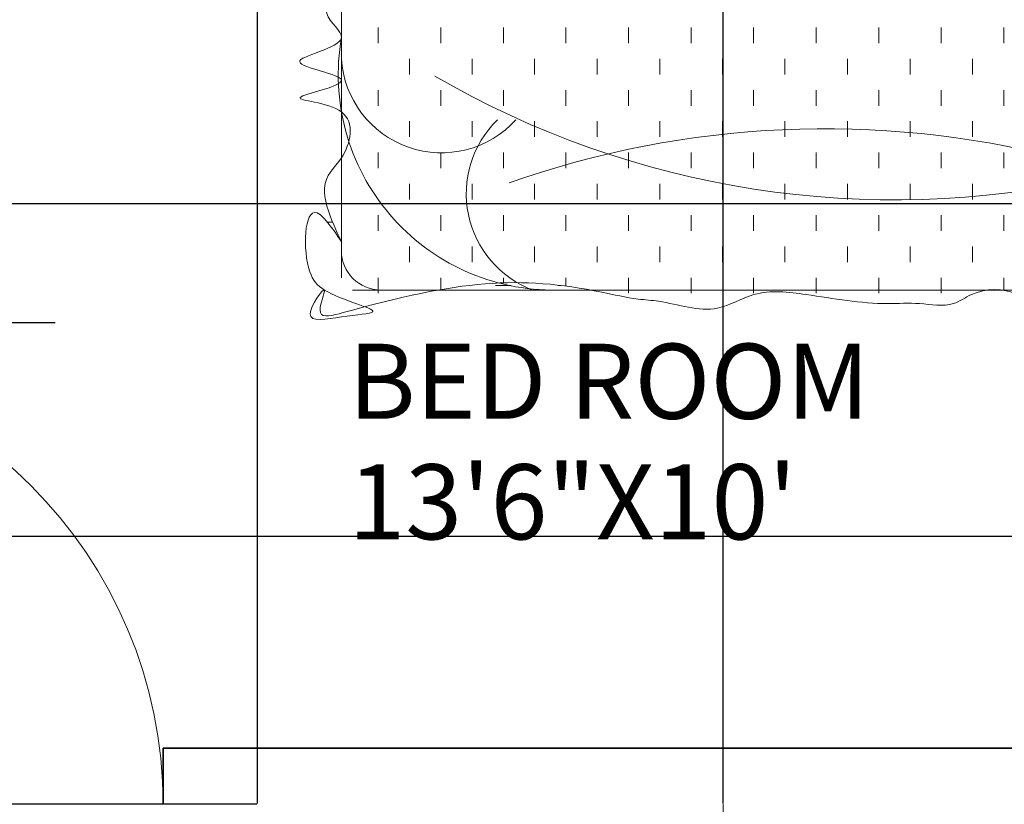
# Model space of a CAD drawing. Units: inches. Extents: x -438 to 102, y -60 to 1091.
# Tile 11 of 20: x -322 to -243, y 898 to 961. Entities that reach past the tile are written whole.
import ezdxf

# ---------------------------------------------------------------- set-up
doc = ezdxf.new("R2010")
doc.units = ezdxf.units.IN
doc.header["$MEASUREMENT"] = 0
for name, color, linetype, lineweight, true_color in [('A-ANNO-DIMS', 217, 'Continuous', 18, 0x93278f), ('A-DOOR', 30, 'Continuous', 18, 0xf26722), ('A-WALL', 2, 'Continuous', 35, 0xf1eb1f)]:
    doc.layers.add(name, color=color, linetype=linetype, lineweight=lineweight, true_color=true_color)
for name, color, linetype, lineweight in [('A-AREA-IDEN', 4, 'Continuous', 18), ('A-FLOR-CASE', 7, 'Continuous', 18), ('Furniture', 7, 'Continuous', 15)]:
    doc.layers.add(name, color=color, linetype=linetype, lineweight=lineweight)
doc.styles.get("Standard").update_dxf_attribs({"font": 'arial.ttf'})
doc.dimstyles.get("Standard").update_dxf_attribs({"dimtxt": 8, "dimasz": 0.18, "dimexe": 0.18, "dimexo": 0.0625, "dimgap": 0.09, "dimtad": 0, "dimtih": 1, "dimtoh": 1, "dimdec": 4, "dimzin": 0, "dimdsep": 46, "dimlunit": 3, "dimtxsty": 'Standard', "dimcen": 0.09, "dimadec": 0, "dimazin": 0, "dimtfac": 1, "dimtdec": 4, "dimtofl": 0, "dimtmove": 0, "dimatfit": 3, "dimfxl": 1, "dimtolj": 1, "dimtzin": 0, "dimarcsym": 0})

# ---------------------------------------------------------------- blocks, each defined once
blk = doc.blocks.new('BED-DOUBLE-WITH-NIGHTSTANDS')
for p, q in [((-29.157, -79.94), (-29.157, -44.493)), ((-26.218, -61.19), (-26.218, -59.94)), ((-21.218, -61.19), (-21.218, -59.94)), ((-16.218, -61.19), (-16.218, -59.94)), ((-11.218, -61.19), (-11.218, -59.94)), ((-6.218, -61.19), (-6.218, -59.94)), ((-1.218, -61.19), (-1.218, -59.94)), ((3.782, -61.19), (3.782, -59.94)), ((8.782, -61.19), (8.782, -59.94)), ((13.782, -61.19), (13.782, -59.94)), ((18.782, -61.19), (18.782, -59.94)), ((23.782, -61.19), (23.782, -59.94)), ((-23.718, -63.69), (-23.718, -62.44)), ((-18.718, -63.69), (-18.718, -62.44)), ((-13.718, -63.69), (-13.718, -62.44)), ((-8.718, -63.69), (-8.718, -62.44)), ((-3.718, -63.69), (-3.718, -62.44)), ((1.282, -63.69), (1.282, -62.44)), ((6.282, -63.69), (6.282, -62.44)), ((11.282, -63.69), (11.282, -62.44)), ((16.282, -63.69), (16.282, -62.44)), ((21.282, -63.69), (21.282, -62.44)), ((-26.218, -66.19), (-26.218, -64.94)), ((-21.218, -66.19), (-21.218, -64.94)), ((-16.218, -66.19), (-16.218, -64.94)), ((-11.218, -66.19), (-11.218, -64.94)), ((-6.218, -66.19), (-6.218, -64.94)), ((-1.218, -66.19), (-1.218, -64.94)), ((3.782, -66.19), (3.782, -64.94)), ((8.782, -66.19), (8.782, -64.94)), ((13.782, -66.19), (13.782, -64.94)), ((18.782, -66.19), (18.782, -64.94)), ((23.782, -66.19), (23.782, -64.94)), ((-23.718, -68.69), (-23.718, -67.44)), ((-18.718, -68.69), (-18.718, -67.44)), ((-13.718, -68.69), (-13.718, -67.44)), ((-8.718, -68.69), (-8.718, -67.44)), ((-3.718, -68.69), (-3.718, -67.44)), ((1.282, -68.69), (1.282, -67.44)), ((6.282, -68.69), (6.282, -67.44)), ((11.282, -68.69), (11.282, -67.44)), ((16.282, -68.69), (16.282, -67.44)), ((21.282, -68.69), (21.282, -67.44)), ((-26.218, -71.19), (-26.218, -69.94)), ((-21.218, -71.19), (-21.218, -69.94)), ((-16.218, -71.19), (-16.218, -69.94)), ((-11.218, -71.19), (-11.218, -69.94)), ((-6.218, -71.19), (-6.218, -69.94)), ((-1.218, -71.19), (-1.218, -69.94)), ((3.782, -71.19), (3.782, -69.94)), ((8.782, -71.19), (8.782, -69.94)), ((13.782, -71.19), (13.782, -69.94)), ((18.782, -71.19), (18.782, -69.94)), ((23.782, -71.19), (23.782, -69.94)), ((-23.718, -73.69), (-23.718, -72.44)), ((-18.718, -73.69), (-18.718, -72.44)), ((-13.718, -73.69), (-13.718, -72.44)), ((-8.718, -73.69), (-8.718, -72.44)), ((-3.718, -73.69), (-3.718, -72.44)), ((1.282, -73.69), (1.282, -72.44)), ((6.282, -73.69), (6.282, -72.44)), ((11.282, -73.69), (11.282, -72.44)), ((16.282, -73.69), (16.282, -72.44)), ((21.282, -73.69), (21.282, -72.44)), ((-29.87, -75.491), (-30.279, -75.491)), ((-26.218, -76.19), (-26.218, -74.94)), ((-21.218, -76.19), (-21.218, -74.94)), ((-16.218, -76.19), (-16.218, -74.94)), ((-11.218, -76.19), (-11.218, -74.94)), ((-6.218, -76.19), (-6.218, -74.94)), ((-1.218, -76.19), (-1.218, -74.94)), ((3.782, -76.19), (3.782, -74.94)), ((8.782, -76.19), (8.782, -74.94)), ((13.782, -76.19), (13.782, -74.94)), ((18.782, -76.19), (18.782, -74.94)), ((23.782, -76.19), (23.782, -74.94)), ((-23.718, -78.69), (-23.718, -77.44)), ((-18.718, -78.69), (-18.718, -77.44)), ((-13.718, -78.69), (-13.718, -77.44)), ((-8.718, -78.69), (-8.718, -77.44)), ((-3.718, -78.69), (-3.718, -77.44)), ((1.282, -78.69), (1.282, -77.44)), ((6.282, -78.69), (6.282, -77.44)), ((11.282, -78.69), (11.282, -77.44)), ((16.282, -78.69), (16.282, -77.44)), ((21.282, -78.69), (21.282, -77.44)), ((-26.218, -81.19), (-26.218, -79.94)), ((-21.218, -80.893), (-21.218, -79.94)), ((-16.218, -80.354), (-16.218, -79.94)), ((-11.218, -80.612), (-11.218, -79.94)), ((-6.218, -81.19), (-6.218, -79.94)), ((-1.218, -81.19), (-1.218, -79.94)), ((3.782, -81.19), (3.782, -79.94)), ((8.782, -81.19), (8.782, -79.94)), ((13.782, -81.19), (13.782, -79.94)), ((18.782, -81.19), (18.782, -79.94)), ((23.782, -80.944), (23.782, -79.94)), ((33.596, -80.928), (-28.288, -80.928)), ((-15.593, -80.565), (-16.843, -80.565)), ((-11.59, -80.565), (-11.843, -80.565))]:
    blk.add_line(p, q)
for centre, radius, start, end in [((-12.201, -63.717), 17.214, 170.06779, 270.93205), ((-21.159, -61.944), 8.013, 183.53609, 317.84857), ((14.986, -0.753), 72.965, 239.8126, 282.54723), ((-10.938, -73.228), 8.244, 134.23532, 249.05847), ((9.498, -143.884), 75.853, 75.71433, 109.44594), ((-26.01, -77.778), 3.15, 180, 270)]:
    blk.add_arc(centre, radius, start, end)
blk.add_open_spline([(30.963, -44.508), (30.926, -45.187), (30.862, -46.385), (29.771, -47.932), (30.68, -49.438), (30.181, -51.195), (31.183, -52.546), (31.556, -54.753), (29.857, -57.224), (32.609, -60.735), (30.283, -61.502), (30.515, -62.875), (30.787, -64.379), (31.375, -66.149), (31.511, -67.951), (30.622, -69.27), (30.889, -70.902), (30.721, -72.32), (31.738, -73.744), (30.928, -75.806), (31.246, -77.781), (31.095, -79.972), (33.091, -80.014), (31.893, -81.001), (31.103, -80.322), (30.205, -81.428), (28.73, -82.665), (26.29, -82.307), (24.174, -80.727), (21.697, -80.779), (19.495, -82.403), (17.064, -81.884), (13.167, -82.166), (8.822, -81.359), (4.068, -80.767), (0.461, -83.087), (-2.79, -81.846), (-5.869, -81.655), (-14.296, -79.687), (-20.145, -80.176), (-31.546, -83.45), (-29.775, -79.604), (-32.809, -83.796), (-29.072, -82.964), (-24.845, -82.73), (-30.357, -81.504), (-32.306, -79.089), (-32.112, -72.198), (-27.723, -79.522), (-31.689, -72.602), (-28.723, -70.506), (-27.651, -65.929), (-35.205, -65.768), (-26.021, -64.125), (-35.787, -62.68), (-27.319, -61.348), (-31.947, -58.401), (-27.389, -55.207), (-31.953, -53.756), (-28.502, -51.755), (-29.554, -48.806), (-29.069, -42.18), (-29.131, -46.294), (-29.157, -48.01)], degree=3, knots=[0, 0, 0, 0, 2.033881, 3.581387, 5.07489, 6.704853, 8.655612, 9.757262, 13.24098, 16.903694, 18.063816, 18.788243, 20.635227, 22.875483, 24.324336, 25.871843, 27.320698, 29.140811, 29.950855, 32.312207, 34.847704, 36.565952, 37.541804, 38.447727, 39.194923, 40.100844, 41.912688, 45.194843, 46.251388, 49.875946, 51.496686, 54.215105, 56.7523, 63.316606, 67.484853, 70.581422, 75.324573, 76.965649, 79.915763, 100.671038, 102.483321, 104.317501, 106.523635, 109.038061, 111.571263, 115.809372, 117.667229, 122.411431, 125.445794, 129.976907, 132.758854, 136.424739, 139.918708, 143.481583, 147.135325, 151.002466, 153.252794, 157.23352, 159.244583, 161.905351, 164.097269, 169.015093, 172.531686, 172.531686, 172.531686, 172.531686])
blk = doc.blocks.new('DOOR-SWING-36')
for p, q in [((-36, 0), (0, 0)), ((-2, 0), (-2, -36)), ((0, 0), (0, -36))]:
    blk.add_line(p, q)
blk.add_arc((0, 0), 36, 180, 270)
blk = doc.blocks.new('*D13')
at = {"layer": 'A-ANNO-DIMS', "color": 0, "lineweight": -2, "transparency": 16777216}
for p, q in [((-319.332, 1020.043), (-335.045, 1020.043)), ((-334.865, 1019.863), (-334.865, 982.496)), ((-334.865, 936.677), (-334.865, 974.044)), ((-319.332, 936.497), (-335.045, 936.497))]:
    blk.add_line(p, q, dxfattribs=at)
at = {"layer": 'A-ANNO-DIMS', "color": 0, "transparency": 16777216}
for points in [[(-334.895, 1019.863), (-334.835, 1019.863), (-334.865, 1020.043)], [(-334.895, 936.677), (-334.835, 936.677), (-334.865, 936.497)]]:
    blk.add_solid(points, dxfattribs=at)
at = {"layer": 'Defpoints', "color": 0, "transparency": 16777216}
for p in [(-334.865, 1020.043), (-319.269, 1020.043), (-319.269, 936.497)]:
    blk.add_point(p, dxfattribs=at)
at = {"layer": 'A-ANNO-DIMS', "color": 0, "transparency": 16777216, "insert": (-334.865, 978.27), "char_height": 8, "attachment_point": 5}
blk.add_mtext('\\A1;6\'-11 1/2" TYP.', dxfattribs=at)
blk = doc.blocks.new('*D41')
at = {"layer": 'A-ANNO-DIMS', "color": 0, "lineweight": -2, "transparency": 16777216}
for p, q in [((-303.146, 898.062), (-303.146, 1079.579)), ((-302.966, 1079.399), (-295.262, 1079.399)), ((-266.116, 1079.399), (-273.821, 1079.399)), ((-265.936, 898.062), (-265.936, 1079.579))]:
    blk.add_line(p, q, dxfattribs=at)
at = {"layer": 'A-ANNO-DIMS', "color": 0, "transparency": 16777216}
for points in [[(-302.966, 1079.429), (-302.966, 1079.369), (-303.146, 1079.399)], [(-266.116, 1079.429), (-266.116, 1079.369), (-265.936, 1079.399)]]:
    blk.add_solid(points, dxfattribs=at)
at = {"layer": 'Defpoints', "color": 0, "transparency": 16777216}
for p in [(-265.936, 1079.399), (-303.146, 897.999), (-265.936, 897.999)]:
    blk.add_point(p, dxfattribs=at)
at = {"layer": 'A-ANNO-DIMS', "color": 0, "transparency": 16777216, "insert": (-284.541, 1079.399), "char_height": 8, "attachment_point": 5}
blk.add_mtext('\\A1;3\'-1"', dxfattribs=at)
blk = doc.blocks.new('*D44')
at = {"layer": 'A-ANNO-DIMS', "color": 0, "lineweight": -2, "transparency": 16777216}
for p, q in [((-64.709, 945.999), (-414.94, 945.999)), ((-414.76, 945.819), (-414.76, 936.936)), ((-414.76, 919.599), (-414.76, 928.483)), ((-64.709, 919.419), (-414.94, 919.419))]:
    blk.add_line(p, q, dxfattribs=at)
at = {"layer": 'A-ANNO-DIMS', "color": 0, "transparency": 16777216}
for points in [[(-414.79, 945.819), (-414.73, 945.819), (-414.76, 945.999)], [(-414.79, 919.599), (-414.73, 919.599), (-414.76, 919.419)]]:
    blk.add_solid(points, dxfattribs=at)
at = {"layer": 'Defpoints', "color": 0, "transparency": 16777216}
for p in [(-64.646, 945.999), (-414.76, 919.419), (-64.646, 919.419)]:
    blk.add_point(p, dxfattribs=at)
at = {"layer": 'A-ANNO-DIMS', "color": 0, "transparency": 16777216, "insert": (-414.76, 932.709), "char_height": 8, "attachment_point": 5}
blk.add_mtext('\\A1;2\'-2 1/2"', dxfattribs=at)
blk = doc.blocks.new('*D56')
at = {"layer": 'A-ANNO-DIMS', "color": 0, "lineweight": -2, "transparency": 16777216}
for p, q in [((-303.209, 897.999), (-414.94, 897.999)), ((-414.76, 897.819), (-414.76, 890.538)), ((-414.76, 874.803), (-414.76, 882.085)), ((-291.603, 874.623), (-414.94, 874.623))]:
    blk.add_line(p, q, dxfattribs=at)
at = {"layer": 'A-ANNO-DIMS', "color": 0, "transparency": 16777216}
for points in [[(-414.79, 897.819), (-414.73, 897.819), (-414.76, 897.999)], [(-414.79, 874.803), (-414.73, 874.803), (-414.76, 874.623)]]:
    blk.add_solid(points, dxfattribs=at)
at = {"layer": 'Defpoints', "color": 0, "transparency": 16777216}
for p in [(-414.76, 897.999), (-303.146, 897.999), (-291.54, 874.623)]:
    blk.add_point(p, dxfattribs=at)
at = {"layer": 'A-ANNO-DIMS', "color": 0, "transparency": 16777216, "insert": (-414.76, 886.311), "char_height": 8, "attachment_point": 5}
blk.add_mtext('\\A1;1\'-11 1/2"', dxfattribs=at)

msp = doc.modelspace()

# ---------------------------------------------------------------- linework, layer by layer
at = {"layer": 'A-FLOR-CASE'}
msp.add_line((-265.93641, 897.99939), (-265.93641, 834.64014), dxfattribs=at)
at = {"layer": 'A-WALL'}
for p, q in [((-187.64649, 902.49939), (-310.7047, 902.49939)), ((-310.7047, 902.49939), (-310.7047, 897.99939))]:
    msp.add_line(p, q, dxfattribs=at)

# ---------------------------------------------------------------- block references
at = {"layer": 'A-DOOR', "rotation": 180}
msp.add_blockref('DOOR-SWING-36', (-346.7047, 897.99939), dxfattribs=at)
at = {"layer": 'Furniture'}
msp.add_blockref('BED-DOUBLE-WITH-NIGHTSTANDS', (-267.285, 1020.04), dxfattribs=at)

# ---------------------------------------------------------------- texts
at = {"layer": 'A-AREA-IDEN'}
for s, p in [('BED ROOM', (-295.88898, 928.81983)), ('13\'6"X10\'', (-295.88898, 919.18136))]:
    msp.add_text(s, height=6, dxfattribs=at).set_placement(p)

# ---------------------------------------------------------------- dimensions: what is measured, and where the dimension line sits
at = {"layer": 'A-ANNO-DIMS'}
dim = msp.add_linear_dim(base=(-265.93641, 1079.39939), p1=(-303.14649, 897.99939), p2=(-265.93641, 897.99939), dimstyle='Standard', override={"dimdec": 1, "dimlfac": 1, "dimrnd": 0, "dimzin": 1, "dimdsep": 46, "dimlunit": 4, "dimfrac": 2}, dxfattribs=at)
dim.commit()
dim.dimension.update_dxf_attribs({"geometry": '*D41', "text_midpoint": (-284.54145, 1079.39939)})
dim = msp.add_linear_dim(base=(-334.86456, 1020.04286), p1=(-319.26918, 936.49708), p2=(-319.26918, 1020.04286), angle=90, text='<> TYP.', dimstyle='Standard', override={"dimdec": 1, "dimlfac": 1, "dimrnd": 0, "dimzin": 1, "dimdsep": 46, "dimlunit": 4, "dimfrac": 2}, dxfattribs=at)
dim.commit()
dim.dimension.update_dxf_attribs({"geometry": '*D13', "text_midpoint": (-334.86456, 978.26997)})
for base, p1, p2, picture, middle in [((-414.76009, 919.41905), (-64.64649, 945.99939), (-64.64649, 919.41905), '*D44', (-414.76009, 932.70922)), ((-414.76009, 897.99939), (-291.54025, 874.62295), (-303.14649, 897.99939), '*D56', (-414.76009, 886.31117))]:
    dim = msp.add_linear_dim(base=base, p1=p1, p2=p2, angle=90, dimstyle='Standard', override={"dimdec": 1, "dimlfac": 1, "dimrnd": 0, "dimzin": 1, "dimdsep": 46, "dimlunit": 4, "dimfrac": 2}, dxfattribs=at)
    dim.commit()
    dim.dimension.update_dxf_attribs({"geometry": picture, "text_midpoint": middle})

doc.saveas('drawing.dxf')
